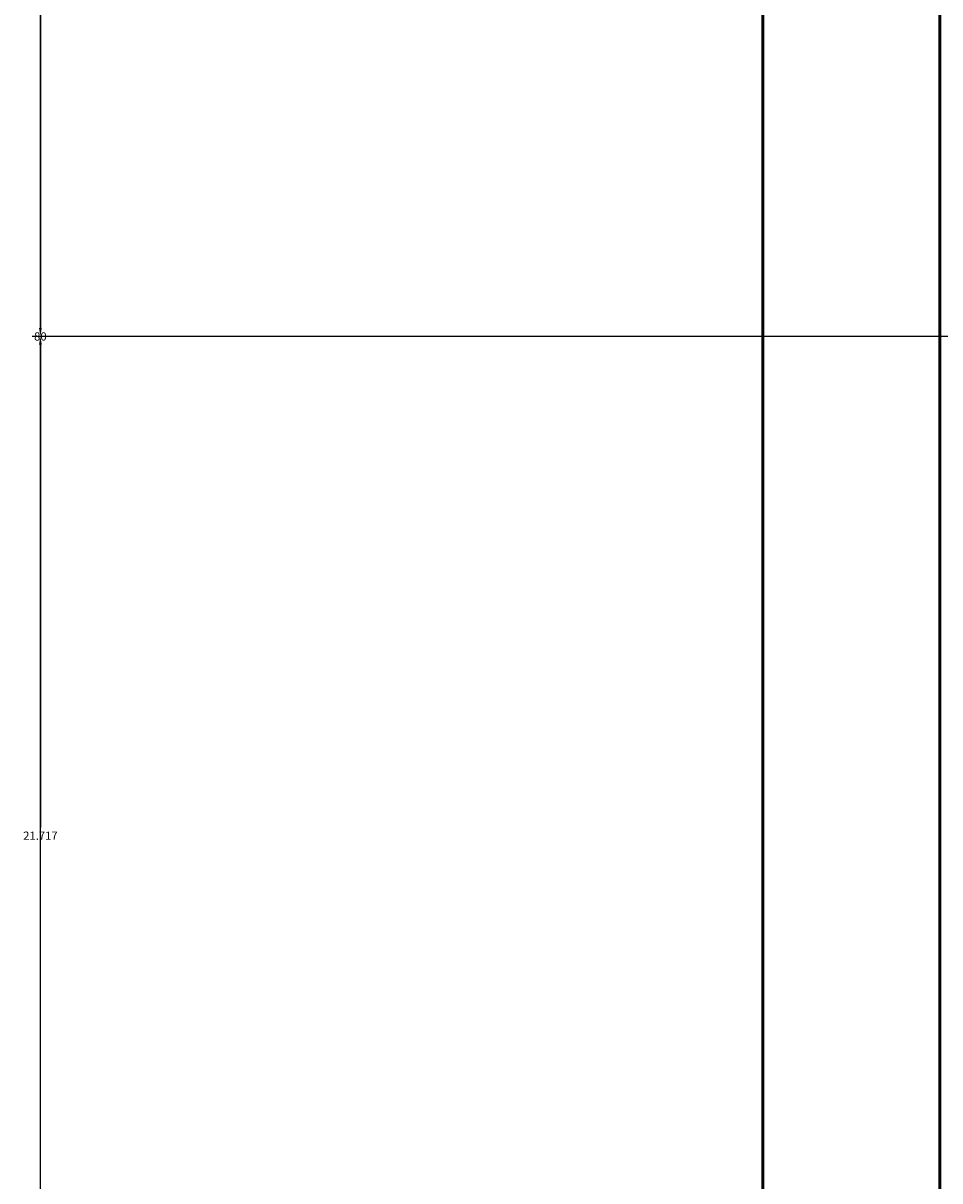
# Model space of a CAD drawing. Units: inches. Extents: x -14 to 108, y -9 to 83.
# Tile 3 of 13: x -14 to 6, y 19 to 44. Entities that reach past the tile are written whole.
import ezdxf

# ---------------------------------------------------------------- set-up
doc = ezdxf.new("R2010")
doc.units = ezdxf.units.IN
doc.header["$MEASUREMENT"] = 0
doc.layers.add('M-DIMS', color=2, linetype='Continuous', lineweight=18)
doc.layers.add('M-OUTL', color=7, linetype='Continuous', lineweight=50)
doc.styles.get("Standard").update_dxf_attribs({"font": 'arial.ttf'})
doc.dimstyles.get("Standard").update_dxf_attribs({"dimtxt": 0.18, "dimasz": 0.18, "dimexe": 0.18, "dimexo": 0.0625, "dimgap": 0.09, "dimtad": 0, "dimtih": 1, "dimtoh": 1, "dimzin": 0, "dimdsep": 46, "dimtxsty": 'Standard', "dimcen": 0.09, "dimadec": 0, "dimazin": 0, "dimtfac": 1, "dimtofl": 0, "dimtmove": 0, "dimatfit": 3, "dimfxl": 1, "dimtolj": 1, "dimtzin": 0, "dimarcsym": 0})

# ---------------------------------------------------------------- blocks, each defined once
blk = doc.blocks.new('SLOT-VERTICAL')
blk.add_lwpolyline([(0, 1.021), (0, 40.458)])
blk = doc.blocks.new('*D5')
at = {"layer": 'Defpoints', "color": 0, "transparency": 16777216}
for p in [(-13.617, 77.119), (2.098, 77.119), (2.098, -2.881)]:
    blk.add_point(p, dxfattribs=at)
at = {"layer": 'M-DIMS', "color": 0, "lineweight": -2, "transparency": 16777216}
for p, q in [((2.035, 77.119), (-13.797, 77.119)), ((-13.617, 76.939), (-13.617, 37.301)), ((-13.617, -2.701), (-13.617, 36.937)), ((2.035, -2.881), (-13.797, -2.881))]:
    blk.add_line(p, q, dxfattribs=at)
at = {"layer": 'M-DIMS', "color": 0, "transparency": 16777216}
for points in [[(-13.647, 76.939), (-13.587, 76.939), (-13.617, 77.119)], [(-13.647, -2.701), (-13.587, -2.701), (-13.617, -2.881)]]:
    blk.add_solid(points, dxfattribs=at)
at = {"layer": 'M-DIMS', "color": 0, "transparency": 16777216, "insert": (-13.617, 37.119), "char_height": 0.18, "attachment_point": 5}
blk.add_mtext('\\A1;80', dxfattribs=at)
blk = doc.blocks.new('*D18')
at = {"layer": 'Defpoints', "color": 0, "transparency": 16777216}
for p in [(-13.617, 55.756), (26.462, 55.756), (16.928, 37.119)]:
    blk.add_point(p, dxfattribs=at)
at = {"layer": 'M-DIMS', "color": 0, "lineweight": -2, "transparency": 16777216}
for p, q in [((26.399, 55.756), (-13.797, 55.756)), ((-13.617, 55.576), (-13.617, 46.619)), ((-13.617, 37.299), (-13.617, 46.256)), ((16.865, 37.119), (-13.797, 37.119))]:
    blk.add_line(p, q, dxfattribs=at)
at = {"layer": 'M-DIMS', "color": 0, "transparency": 16777216}
for points in [[(-13.647, 55.576), (-13.587, 55.576), (-13.617, 55.756)], [(-13.647, 37.299), (-13.587, 37.299), (-13.617, 37.119)]]:
    blk.add_solid(points, dxfattribs=at)
at = {"layer": 'M-DIMS', "color": 0, "transparency": 16777216, "insert": (-13.617, 46.437), "char_height": 0.18, "attachment_point": 5}
blk.add_mtext('\\A1;18.636', dxfattribs=at)
blk = doc.blocks.new('*D19')
at = {"layer": 'Defpoints', "color": 0, "transparency": 16777216}
for p in [(-13.617, 37.119), (16.928, 37.119), (27.381, 15.402)]:
    blk.add_point(p, dxfattribs=at)
at = {"layer": 'M-DIMS', "color": 0, "lineweight": -2, "transparency": 16777216}
for p, q in [((16.865, 37.119), (-13.797, 37.119)), ((-13.617, 36.939), (-13.617, 26.441)), ((-13.617, 15.582), (-13.617, 26.08)), ((27.318, 15.402), (-13.797, 15.402))]:
    blk.add_line(p, q, dxfattribs=at)
at = {"layer": 'M-DIMS', "color": 0, "transparency": 16777216}
for points in [[(-13.647, 36.939), (-13.587, 36.939), (-13.617, 37.119)], [(-13.647, 15.582), (-13.587, 15.582), (-13.617, 15.402)]]:
    blk.add_solid(points, dxfattribs=at)
at = {"layer": 'M-DIMS', "color": 0, "transparency": 16777216, "insert": (-13.617, 26.261), "char_height": 0.18, "attachment_point": 5}
blk.add_mtext('\\A1;21.717', dxfattribs=at)

msp = doc.modelspace()

# ---------------------------------------------------------------- linework, layer by layer
at = {"layer": 'M-OUTL'}
msp.add_lwpolyline([(2.0979, 57.1193), (2.0979, 17.1193)], dxfattribs=at)

# ---------------------------------------------------------------- block references
msp.add_blockref('SLOT-VERTICAL', (5.9511, 17.206), dxfattribs=at)

# ---------------------------------------------------------------- dimensions: what is measured, and where the dimension line sits
at = {"layer": 'M-DIMS'}
for base, p1, p2, override, picture, middle in [((-13.6171, 77.1193), (2.0979, -2.8807), (2.0979, 77.1193), {"dimdec": 0, "dimlfac": 1, "dimrnd": 0, "dimzin": 0, "dimdsep": 46, "dimlunit": 2}, '*D5', (-13.6171, 37.1193)), ((-13.6171, 55.7556), (16.9278, 37.1193), (26.4616, 55.7556), {"dimdec": 3, "dimlfac": 1, "dimrnd": 0, "dimzin": 0, "dimdsep": 46, "dimlunit": 2}, '*D18', (-13.6171, 46.4375)), ((-13.6171, 37.1193), (27.3809, 15.4023), (16.9278, 37.1193), {"dimdec": 3, "dimlfac": 1, "dimrnd": 0, "dimzin": 0, "dimdsep": 46, "dimlunit": 2}, '*D19', (-13.6171, 26.2608))]:
    dim = msp.add_linear_dim(base=base, p1=p1, p2=p2, angle=90, dimstyle='Standard', override=override, dxfattribs=at)
    dim.commit()
    dim.dimension.update_dxf_attribs({"geometry": picture, "text_midpoint": middle})

doc.saveas('drawing.dxf')
